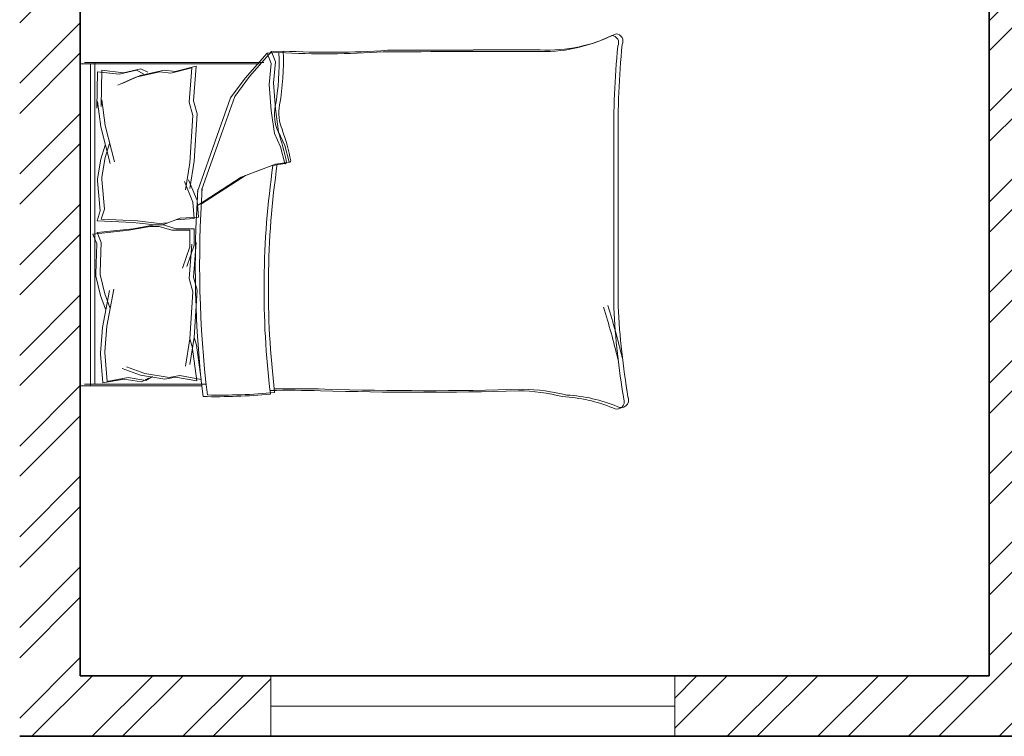
# Model space of a CAD drawing. Units: inches. Extents: x 2120 to 4013, y 1390 to 3019.
# Tile 17 of 59: x 2716 to 2862, y 1582 to 1688. Entities that reach past the tile are written whole.
import ezdxf

# ---------------------------------------------------------------- set-up
doc = ezdxf.new("R2010")
doc.units = ezdxf.units.IN
for name, color, linetype, lineweight in [('A-FURN', 8, 'Continuous', 13), ('A-GLAZ', 4, 'Continuous', 18), ('A-WALL', 7, 'Continuous', 35), ('A-WALL-PATT', 252, 'Continuous', 13)]:
    doc.layers.add(name, color=color, linetype=linetype, lineweight=lineweight)

# ---------------------------------------------------------------- blocks, each defined once
blk = doc.blocks.new('BED-DOUBLE-PLAN')
for p, q in [((3.48, 63.34), (3.48, 81.45)), ((3.48, 81.45), (51.27, 81.45)), ((3.7, 62.7), (3.7, 80.81)), ((51.27, 81.45), (51.27, 54.84)), ((51.5, 80.81), (51.5, 54.2)), ((3.48, 79.91), (51.27, 79.91)), ((3.7, 79.27), (51.5, 79.27)), ((16.88, 78.42), (19.77, 79.14)), ((19.77, 79.14), (20.09, 79.14)), ((20.09, 79.14), (24.54, 79)), ((24.54, 79), (25.98, 79.58)), ((25.98, 79.58), (26.56, 74.23)), ((50.11, 78.89), (44.71, 78.99)), ((44.71, 78.99), (45.71, 78.9)), ((3.9, 78.11), (8.18, 78.44)), ((3.9, 78.13), (4.47, 74.95)), ((4.13, 77.47), (8.41, 77.8)), ((8.18, 78.44), (8.29, 78.42)), ((8.29, 78.42), (12.11, 78.13)), ((8.41, 77.8), (8.51, 77.78)), ((8.51, 77.78), (12.34, 77.49)), ((12.11, 78.13), (17.6, 77.12)), ((14.86, 77.7), (16.88, 78.42)), ((15.08, 77.06), (17.11, 77.78)), ((17.11, 77.78), (20, 78.5)), ((20, 78.5), (20.32, 78.5)), ((20.32, 78.5), (24.77, 78.36)), ((24.77, 78.36), (26.21, 78.94)), ((26.21, 78.94), (26.79, 73.59)), ((27.98, 78.95), (27.73, 73.58)), ((28.21, 78.32), (27.96, 72.94)), ((29.46, 78.47), (27.98, 78.95)), ((29.69, 77.83), (28.21, 78.32)), ((33.89, 78.89), (29.46, 78.47)), ((34.11, 78.25), (29.69, 77.83)), ((34.21, 78.91), (33.89, 78.89)), ((34.43, 78.27), (34.11, 78.25)), ((37.14, 78.37), (34.21, 78.91)), ((37.37, 77.73), (34.43, 78.27)), ((41.92, 78.38), (36.5, 77.02)), ((42.14, 77.74), (36.72, 76.38)), ((39.2, 77.77), (37.14, 78.37)), ((39.43, 77.13), (37.37, 77.73)), ((45.71, 78.9), (41.92, 78.38)), ((45.94, 78.26), (42.14, 77.74)), ((50.34, 78.25), (44.94, 78.35)), ((44.94, 78.35), (45.94, 78.26)), ((50.11, 78.89), (49.73, 75.68)), ((50.34, 78.25), (49.96, 75.04)), ((4.12, 77.49), (4.7, 74.31)), ((12.34, 77.49), (17.83, 76.48)), ((4.47, 74.95), (4.04, 72.35)), ((5.05, 72.49), (6.06, 75.24)), ((5.28, 71.85), (6.29, 74.6)), ((49.31, 73.19), (48.13, 75.87)), ((49.54, 72.55), (48.36, 75.23)), ((49.73, 75.68), (50.33, 73.11)), ((49.96, 75.04), (50.56, 72.47)), ((4.7, 74.31), (4.27, 71.71)), ((26.56, 74.23), (27.14, 71.05)), ((26.79, 73.59), (27.37, 70.41)), ((27.73, 73.58), (27.36, 70.37)), ((50.11, 69.62), (49.31, 73.19)), ((4.04, 72.35), (4.62, 71.33)), ((4.27, 71.71), (4.85, 70.7)), ((4.47, 68.88), (5.05, 72.49)), ((4.7, 68.24), (5.28, 71.85)), ((27.96, 72.94), (27.58, 69.73)), ((50.34, 68.98), (49.54, 72.55)), ((50.33, 73.11), (49.82, 72.06)), ((50.56, 72.47), (50.04, 71.42)), ((27.14, 71.05), (27.14, 69.74)), ((27.36, 70.37), (27.44, 69.07)), ((27.37, 70.41), (27.37, 69.1)), ((4.76, 67.29), (4.47, 68.88)), ((27.14, 69.74), (26.56, 67.86)), ((27.37, 69.1), (26.79, 67.23)), ((27.44, 69.07), (28.13, 67.23)), ((27.58, 69.73), (27.67, 68.43)), ((49.92, 68.01), (50.11, 69.62)), ((50.15, 67.37), (50.34, 68.98)), ((4.19, 64.11), (4.76, 67.29)), ((4.99, 66.65), (4.7, 68.24)), ((26.56, 67.86), (26.56, 65.18)), ((27.67, 68.43), (28.36, 66.59)), ((50.7, 64.87), (49.92, 68.01)), ((50.93, 64.23), (50.15, 67.37)), ((4.41, 63.47), (4.99, 66.65)), ((6.38, 65.82), (10.42, 65.15)), ((24.1, 65.18), (20.96, 66.27)), ((26.79, 67.23), (26.79, 64.54)), ((28.13, 67.23), (28.3, 64.55)), ((28.36, 66.59), (28.53, 63.91)), ((30.75, 64.71), (33.82, 65.99)), ((32.57, 65.82), (36.6, 65.15)), ((9.28, 64.83), (4.19, 64.11)), ((6.61, 65.18), (10.64, 64.51)), ((10.42, 65.15), (9.28, 64.83)), ((10.64, 64.51), (9.51, 64.19)), ((10.42, 65.15), (17.43, 64.72)), ((10.64, 64.51), (17.65, 64.08)), ((17.43, 64.72), (19.39, 65.28)), ((17.65, 64.08), (19.61, 64.64)), ((19.39, 65.28), (24.52, 64.87)), ((19.61, 64.64), (24.75, 64.23)), ((24.33, 64.54), (21.19, 65.63)), ((26.56, 65.18), (24.1, 65.18)), ((26.79, 64.54), (24.33, 64.54)), ((28.3, 64.55), (30.75, 64.71)), ((30.98, 64.07), (34.05, 65.35)), ((32.79, 65.18), (36.83, 64.51)), ((36.6, 65.15), (43.61, 64.72)), ((36.83, 64.51), (43.84, 64.08)), ((43.61, 64.72), (45.57, 65.28)), ((43.84, 64.08), (45.8, 64.64)), ((45.57, 65.28), (50.7, 64.87)), ((45.8, 64.64), (50.93, 64.23)), ((9.51, 64.19), (4.41, 63.47)), ((28.53, 63.91), (30.98, 64.07)), ((30.26, 64.06), (34.45, 57.57)), ((30.49, 63.42), (34.68, 56.93)), ((40.65, 61.13), (32.31, 64.06)), ((40.87, 60.49), (32.54, 63.42)), ((46.22, 59.12), (40.65, 61.13)), ((46.45, 58.48), (40.87, 60.49)), ((49.16, 56.95), (46.22, 59.12)), ((34.45, 57.57), (36.15, 53.08)), ((49.39, 56.31), (46.45, 58.48)), ((34.68, 56.93), (36.38, 52.44)), ((52.87, 53.7), (49.16, 56.95)), ((53.1, 53.06), (49.39, 56.31)), ((36.15, 53.08), (36.46, 51.07)), ((40.96, 52.62), (44.36, 53.08)), ((44.36, 53.08), (48.23, 53.39)), ((44.59, 52.44), (48.46, 52.75)), ((48.23, 53.39), (51.33, 53.08)), ((48.46, 52.75), (51.56, 52.44)), ((51.33, 53.08), (52.87, 53.7)), ((51.56, 52.44), (53.1, 53.06)), ((52.95, 51.96), (52.87, 53.7, 3.87)), ((53.18, 51.32), (53.1, 53.06, 3.87)), ((36.38, 52.44), (36.69, 50.43)), ((36.46, 51.07), (38.94, 51.69)), ((38.94, 51.69), (40.96, 52.62)), ((39.17, 51.05), (41.18, 51.98)), ((41.18, 51.98), (44.59, 52.44)), ((36.69, 50.43), (39.17, 51.05)), ((15.06, 2.2), (39.68, 2.2)), ((15.29, 1.56), (39.91, 1.56))]:
    blk.add_line(p, q)
for centre, radius, start, end in [((21.36, -100.61), 164.97, 86.0865, 96.7821), ((85.16, 61.35), 83.31, 178.7218, 185.604), ((21.59, -101.25), 164.97, 86.0865, 96.7821), ((85.39, 60.71), 83.31, 178.7218, 185.604), ((17.76, -74.87), 129.02, 81.7845, 96.9006), ((17.99, -75.51), 129.02, 81.7845, 96.9006), ((-167.31, 50.27), 170.11, 358.4762, 1.0082), ((-167.08, 49.63), 170.11, 358.4762, 1.0082), ((31.16, 79.96), 29.65, 280.6617, 289.8806), ((31.38, 79.32), 29.65, 280.6617, 289.8806), ((43.74, 46.38), 6.22, 78.6608, 113.7384), ((43.97, 45.74), 6.22, 78.6608, 113.7384), ((51.33, 88.1), 36.18, 259.8763, 272.5657), ((51.56, 87.46), 36.18, 259.8763, 272.5657), ((182.27, 45.13), 129.5, 176.9791, 183.8365), ((182.5, 44.49), 129.5, 176.9791, 183.8365), ((36.64, 51.01), 0.185, 160.2464, 271.1377), ((36.87, 50.37), 0.185, 160.2464, 271.1377), ((484.82, 30.83), 482.31, 178.2277, 181.7185), ((485.05, 30.19), 482.31, 178.2277, 181.7185), ((-4508.74, 13.62), 4561.86, 0.00217, 0.28689), ((-4508.51, 12.99), 4561.86, 0.00217, 0.28689), ((-26.9, 16.93), 29.63, 346.0648, 358.9113), ((-26.67, 16.29), 29.63, 346.0648, 358.9113), ((76.16, 12.78), 23.07, 177.4714, 206.4681), ((76.39, 12.14), 23.07, 177.4714, 206.4681), ((-21.66, 11.17), 23.56, 337.9751, 356.652), ((-21.43, 10.53), 23.56, 337.9751, 356.652), ((-17.22, 105.16), 106.46, 283.3832, 287.7053), ((-16.99, 104.52), 106.46, 283.3832, 287.7053), ((1.09, 1.73), 1.09, 146.1736, 293.4781), ((1.32, 1.09), 1.09, 146.1736, 293.4781), ((21.43, -119.39), 121.76, 92.9958, 99.4091), ((21.66, -120.03), 121.76, 92.9958, 99.4091), ((41.15, -130.83), 133.04, 84.4998, 90.6351), ((41.38, -131.47), 133.04, 84.4998, 90.6351), ((54.41, 2.58), 1.1, 242.6588, 356.02), ((54.64, 1.94), 1.1, 242.6588, 356.02)]:
    blk.add_arc(centre, radius, start, end)
blk = doc.blocks.new('WIN-PLAN-60IN-04')
for p, q in [((0, 9), (0, 9)), ((0, 9), (0, 0)), ((60, 4.5), (60, 9)), ((60, 9), (60, 0)), ((0, 0), (0, 4.5)), ((0, 4.5), (60, 4.5))]:
    blk.add_line(p, q)

msp = doc.modelspace()

# ---------------------------------------------------------------- hatches: boundary and pattern name
at = {"layer": 'A-WALL-PATT'}
h = msp.add_hatch(dxfattribs=at)
h.set_pattern_fill('ANSI32', color=256)
h.paths.add_polyline_path([(2271.7331, 2122.6377), (2262.7331, 2122.6377), (2262.7331, 2040.3893), (2267.2331, 2040.3893), (2271.7331, 2040.3893), (2271.7331, 2044.8856), (2271.7331, 2070.531), (2391.7331, 2070.531), (2391.7331, 1926.5306), (2388.3993, 1926.5306), (2388.3993, 1922.531), (2395.7331, 1922.531), (2395.7331, 1992.531), (2400.4511, 1992.531), (2400.4511, 1997.0306), (2395.7331, 1997.0306), (2395.7331, 2070.531), (2443.7331, 2070.531), (2443.7331, 2046.1368), (2448.2331, 2046.1368), (2448.2331, 2070.531), (2580.2331, 2070.531), (2580.2331, 1997.0306), (2492.9076, 1997.0306), (2492.9076, 1992.531), (2580.2331, 1992.531), (2580.2331, 1983.9368), (2589.2331, 1983.9368), (2589.2331, 2070.531), (2589.2331, 2075.0306), (2396.2331, 2075.0306), (2396.2331, 2184.3565), (2393.9831, 2184.3565), (2391.7331, 2184.3565), (2391.7331, 2075.0306), (2271.7331, 2075.0306)])
h.paths.add_polyline_path([(2724.7331, 2138.0306), (2628.7331, 2138.0306), (2628.7331, 2070.5306), (2628.7331, 2067.0987), (2633.2331, 2067.0987), (2637.7331, 2067.0987), (2637.7331, 2070.531), (2657.3413, 2070.531), (2657.3413, 2079.5306), (2637.7331, 2079.5306), (2637.7331, 2129.031), (2715.7331, 2129.031), (2715.7331, 2079.5306), (2698.0378, 2079.5306), (2698.0378, 2070.531), (2715.7331, 2070.531), (2715.7331, 2012.1531), (2720.2331, 2012.1531), (2724.7331, 2012.1531)])
h.paths.add_polyline_path([(2724.7331, 2213.031), (2831.3209, 2213.031), (2831.3209, 2215.281), (2831.3209, 2217.5306), (2724.7331, 2217.5306), (2724.7331, 2343.531), (2751.8755, 2343.531), (2751.8755, 2352.5306), (2715.7331, 2352.5306), (2715.7331, 2138.031), (2724.7331, 2138.031)])
h.paths.add_polyline_path([(2902.53, 2352.5306), (2811.8755, 2352.5306), (2811.8755, 2343.531), (2867.2331, 2343.531), (2867.2331, 2217.5306), (2863.6364, 2217.5306), (2863.6364, 2213.031), (2871.7331, 2213.031), (2871.7331, 2217.531), (2871.7331, 2343.531), (2902.53, 2343.531)])
h.paths.add_polyline_path([(3009.7331, 2352.5306), (2938.53, 2352.5306), (2938.53, 2343.531), (2966.2331, 2343.531), (2966.2331, 2242.3281), (2968.4831, 2242.3281), (2970.7331, 2242.3281), (2970.7331, 2343.531), (3009.7331, 2343.531)])
h.paths.add_polyline_path([(3009.7331, 2217.5306), (2970.7331, 2217.5306), (2970.7331, 2220.5422), (2968.4831, 2220.5422), (2966.2331, 2220.5422), (2966.2331, 2217.5306), (2911.7752, 2217.5306), (2907.7331, 2217.5306), (2907.7331, 2213.0306), (2907.7331, 2194.9663), (2912.2331, 2194.9663), (2912.2331, 2213.031), (2970.7331, 2213.031), (3000.7331, 2213.031), (3000.7331, 2205.523), (3009.7331, 2205.523)])
h.paths.add_polyline_path([(3009.7331, 2181.5227), (3000.7331, 2181.5227), (3000.7331, 2165.0306), (2912.2331, 2165.0306), (2912.2331, 2170.8202), (2907.7331, 2170.8202), (2907.7331, 2165.0306), (2899.5169, 2165.0306), (2899.5169, 2162.7806), (2899.5169, 2160.531), (2907.7331, 2160.531), (2907.7331, 2137.3432), (2912.2331, 2137.3432), (2912.2331, 2160.531), (3000.7331, 2160.531), (3000.7331, 2150.4993), (3009.7331, 2150.4993)])
h.paths.add_polyline_path([(3009.7331, 2126.499), (3005.2331, 2126.499), (3000.7331, 2126.499), (3000.7331, 2112.5306), (2912.2331, 2112.5306), (2912.2331, 2115.6036), (2907.7331, 2115.6036), (2907.7331, 2108.031), (3000.7331, 2108.031), (3000.7331, 2084.7256), (3009.7331, 2084.7256)], flags=17)
h.paths.add_polyline_path([(3009.7331, 1971.531), (3009.7331, 2024.7253), (3000.7331, 2024.7253), (3000.7331, 2006.4153), (3000.7331, 1971.5306), (2864.2331, 1971.5306), (2864.2331, 2160.531), (2868.0522, 2160.531), (2868.0522, 2165.0306), (2859.7331, 2165.0306), (2859.7331, 1971.5306), (2724.7331, 1971.5306), (2724.7331, 1977.7012), (2715.7331, 1977.7012), (2715.7331, 1962.5306), (2715.7331, 1950.9035), (2720.2331, 1950.9035), (2724.7331, 1950.9035), (2724.7331, 1962.531), (2855.2331, 1962.531), (2859.7331, 1962.531), (2859.7331, 1835.031), (2864.2331, 1834.8158), (2864.2331, 1962.531), (2958.7331, 1962.531), (2958.7331, 1937.0925), (2963.2331, 1937.0925), (2963.2331, 1962.531), (3000.7331, 1962.531), (3009.7331, 1962.531)])
h.paths.add_polyline_path([(2724.7331, 1728.531), (2822.7164, 1728.531), (2822.7164, 1733.0306), (2724.7331, 1733.0306), (2724.7331, 1779.3416), (2715.7331, 1779.3416), (2715.7331, 1581.531), (2753.02, 1581.531), (2753.02, 1586.031), (2753.02, 1590.5306), (2724.7331, 1590.5306)])
h.paths.add_polyline_path([(2864.2331, 1590.531), (2864.2331, 1787.031), (2868.4075, 1787.031), (2868.4075, 1791.5306), (2859.7331, 1791.5306), (2859.7331, 1739.0306), (2859.7331, 1733.0306), (2854.3125, 1733.0306), (2854.3125, 1728.531), (2859.7331, 1728.531), (2859.7331, 1590.5306), (2813.02, 1590.5306), (2813.02, 1581.531), (2868.4123, 1581.531), (2868.4123, 1583.781), (2868.4123, 1586.0306), (2864.2331, 1586.0306)])
h.paths.add_polyline_path([(3009.7331, 1754.6619), (3000.7331, 1754.6619), (3000.7331, 1739.0306), (2912.2331, 1739.0306), (2912.2331, 1742.2257), (2907.7331, 1742.2257), (2907.7331, 1739.0306), (2907.7331, 1734.531), (3000.7331, 1734.531), (3000.7331, 1590.5306), (3000.7331, 1586.0306), (2971.3921, 1586.0306), (2971.3921, 1581.531), (3009.7331, 1581.531)])
h.paths.add_polyline_path([(2911.3921, 1583.781), (2911.3921, 1586.0306), (2891.2138, 1586.0306), (2891.2138, 1581.531), (2911.3921, 1581.531)])
h.paths.add_polyline_path([(3009.7331, 1799.8422), (3000.7331, 1799.8422), (3000.7331, 1791.5306), (2912.2331, 1791.5306), (2912.2331, 1796.3264), (2909.9831, 1796.3264), (2907.7331, 1796.3264), (2907.7331, 1791.5306), (2902.7033, 1791.5306), (2902.7033, 1787.031), (2907.7331, 1787.031), (2907.7331, 1761.1622), (2912.2331, 1761.1622), (2912.2331, 1787.031), (3000.7331, 1787.031), (3000.7331, 1778.6622), (3009.7331, 1778.6622)])
h.paths.add_polyline_path([(3009.7331, 1839.5306), (2963.2331, 1839.5306), (2963.2331, 1842.8629), (2960.9831, 1842.8629), (2958.7331, 1842.8629), (2958.7331, 1839.5306), (2907.7331, 1839.5306), (2907.7331, 1814.4599), (2912.2331, 1814.4599), (2912.2331, 1835.031), (3000.7331, 1835.031), (3000.7331, 1823.8425), (3009.7331, 1823.8425), (3009.7331, 1835.031)])
h.paths.add_polyline_path([(2963.2331, 1901.0922), (2960.9831, 1901.0922), (2958.7331, 1901.0922), (2958.7331, 1862.8843), (2963.2331, 1862.8843)], flags=17)
h.paths.add_polyline_path([(2724.7331, 1891.9826), (2724.7331, 1914.3416), (2715.7331, 1914.3416), (2715.7331, 1783.8416), (2637.7331, 1783.8416), (2637.7331, 1914.3416), (2628.7331, 1914.3416), (2624.7701, 1914.3416), (2624.7701, 1909.8416), (2624.7701, 1905.3419), (2628.7331, 1905.3419), (2628.7331, 1876.9915), (2628.7331, 1779.3419), (2637.7331, 1779.3419), (2715.7331, 1779.3419), (2724.7331, 1779.3419), (2724.7331, 1835.031)])
h.paths.add_polyline_path([(2637.7331, 1731.531), (2637.7331, 1779.3416), (2628.7331, 1779.3416), (2628.7331, 1731.5306), (2589.2331, 1731.5306), (2535.9814, 1731.5306), (2496.7331, 1731.5306), (2496.7331, 1725.6876), (2498.9831, 1725.6876), (2501.2331, 1725.6876), (2501.2331, 1727.031), (2628.7331, 1727.031), (2628.7331, 1680.4203), (2628.7331, 1590.5306), (2628.7331, 1586.0306), (2604.1361, 1586.0306), (2604.1361, 1581.531), (2637.7331, 1581.531), (2637.7331, 1590.531)])

# ---------------------------------------------------------------- linework, layer by layer
at = {"layer": 'A-WALL'}
for p, q in [((2724.7331, 1590.531), (2724.7331, 1728.531)), ((2724.7331, 1590.531), (2724.7331, 1728.531)), ((2724.7331, 1590.5306), (2724.7331, 1728.5306)), ((2724.7331, 1590.5306), (2724.7331, 1728.5306)), ((2859.7331, 1590.531), (2859.7331, 1728.531)), ((2859.7331, 1590.5306), (2859.7331, 1728.5306)), ((2859.7331, 1590.531), (2724.7331, 1590.531)), ((2859.7331, 1590.5306), (2724.7331, 1590.5306)), ((2870.4123, 1581.531), (2715.7331, 1581.531)), ((2870.4124, 1581.5306), (2715.7331, 1581.5306))]:
    msp.add_line(p, q, dxfattribs=at)

# ---------------------------------------------------------------- block references
at = {"layer": 'A-FURN'}
for p, rotation in [((2806.1794, 1630.12), 90.00000000000003), ((2806.1794, 1630.1197), 89.99999999999999)]:
    msp.add_blockref('BED-DOUBLE-PLAN', p, dxfattribs=dict(at, rotation=rotation))
at = {"layer": 'A-GLAZ'}
for p in [(2753.02, 1581.531), (2753.02, 1581.5306)]:
    msp.add_blockref('WIN-PLAN-60IN-04', p, dxfattribs=at)

doc.saveas('drawing.dxf')
